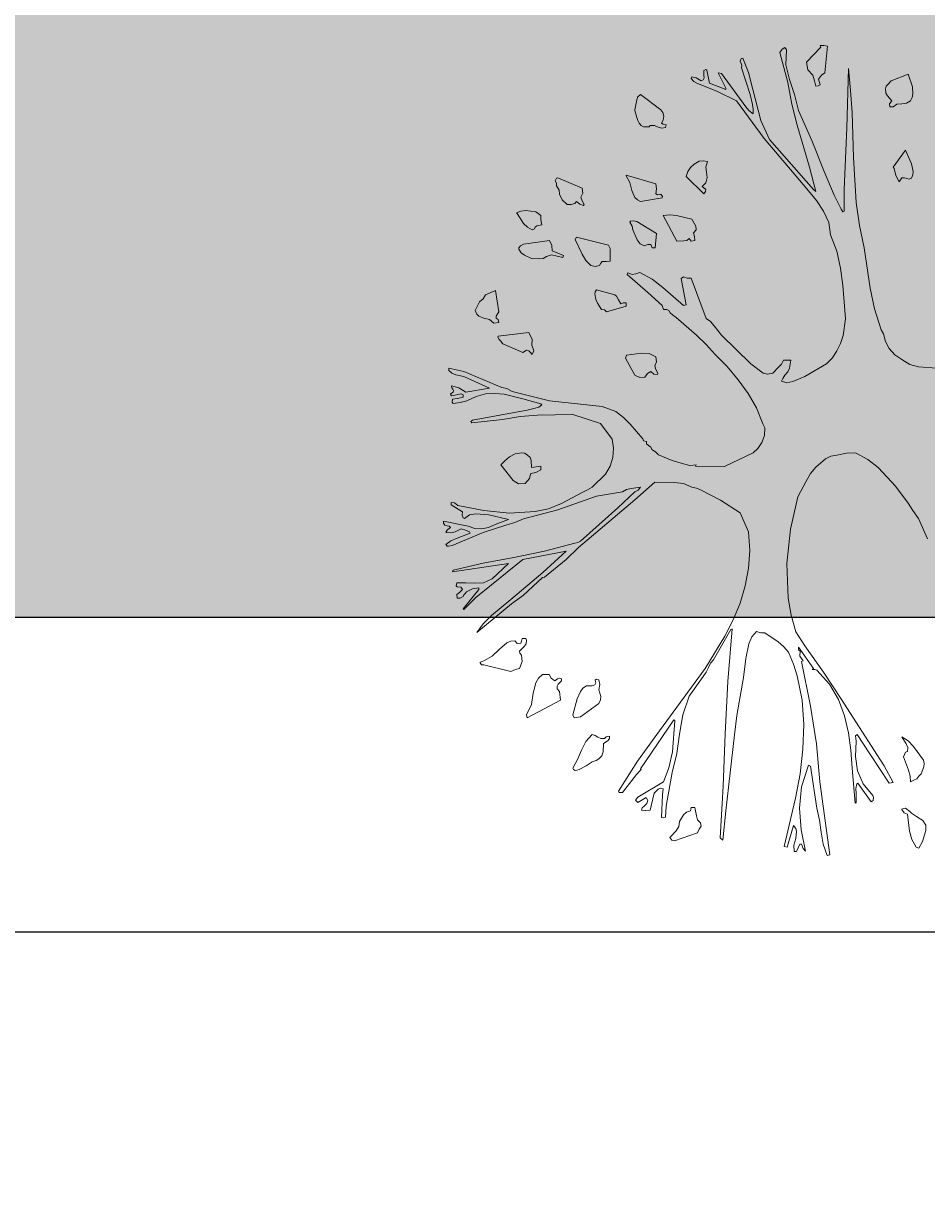
# Model space of a CAD drawing. Units: inches. Extents: x 84 to 1044, y -280 to 906.
# Tile 41 of 105: x 915 to 941, y -129 to -96. Entities that reach past the tile are written whole.
import ezdxf

# ---------------------------------------------------------------- set-up
doc = ezdxf.new("R2010")
doc.units = ezdxf.units.IN
for name, color, linetype, lineweight in [('A-ANNO-DIMS', 2, 'Continuous', 18), ('C-PROP', 7, 'Continuous', 25), ('L-PLNT', 114, 'Continuous', 15)]:
    doc.layers.add(name, color=color, linetype=linetype, lineweight=lineweight)
doc.layers.add('L-PLNT-PATT', color=9, linetype='Continuous', lineweight=9, true_color=0xafd9aa)
doc.styles.get("Standard").update_dxf_attribs({"font": 'arial.ttf'})
doc.dimstyles.get("Standard").update_dxf_attribs({"dimtxt": 0.18, "dimasz": 0.18, "dimexe": 0.18, "dimexo": 0.0625, "dimgap": 0.09, "dimtad": 0, "dimtih": 1, "dimtoh": 1, "dimdec": 4, "dimzin": 0, "dimdsep": 46, "dimtxsty": 'Standard', "dimcen": 0.09, "dimadec": 0, "dimazin": 0, "dimtfac": 1, "dimtdec": 4, "dimtofl": 0, "dimtmove": 0, "dimatfit": 3, "dimfxl": 1, "dimtolj": 1, "dimtzin": 0, "dimarcsym": 0})

# ---------------------------------------------------------------- blocks, each defined once
blk = doc.blocks.new('A$C37E508DF')
for p, q in [((0.6367, 1.5175), (0.6423, 1.5201)), ((0.6423, 1.5201), (0.6453, 1.5158)), ((0.6826, 1.493), (0.7096, 1.5209)), ((0.7083, 1.5239), (0.7152, 1.5244)), ((0.7096, 1.5209), (0.7083, 1.5239)), ((0.7152, 1.5244), (0.7225, 1.5231)), ((0.7225, 1.5231), (0.7174, 1.4729)), ((0.5583, 1.4948), (0.5596, 1.4995)), ((0.5596, 1.4995), (0.563, 1.5003)), ((0.563, 1.5003), (0.5737, 1.4733)), ((0.6329, 1.5111), (0.6367, 1.5175)), ((0.6475, 1.4545), (0.6329, 1.5111)), ((0.6453, 1.5158), (0.644, 1.4879)), ((0.4897, 1.4772), (0.4935, 1.4789)), ((0.4897, 1.4678), (0.4897, 1.4772)), ((0.4935, 1.4789), (0.4952, 1.478)), ((0.4952, 1.478), (0.5004, 1.4532)), ((0.5596, 1.4905), (0.5583, 1.4948)), ((0.5613, 1.4862), (0.5596, 1.4905)), ((0.5608, 1.4823), (0.5613, 1.4862)), ((0.5767, 1.4317), (0.5608, 1.4823)), ((0.644, 1.4879), (0.6505, 1.46)), ((0.6852, 1.4785), (0.6826, 1.493)), ((0.6946, 1.4682), (0.6852, 1.4785)), ((0.7589, 1.3691), (0.7615, 1.481)), ((0.7615, 1.481), (0.7658, 1.4395)), ((0.4657, 1.4622), (0.4669, 1.4652)), ((0.4708, 1.4566), (0.4657, 1.4622)), ((0.4669, 1.4652), (0.4755, 1.463)), ((0.4764, 1.4532), (0.4708, 1.4566)), ((0.4755, 1.463), (0.4845, 1.4575)), ((0.5154, 1.4373), (0.4764, 1.4532)), ((0.4845, 1.4575), (0.4884, 1.4596)), ((0.4884, 1.4596), (0.4905, 1.4635)), ((0.4905, 1.4635), (0.4897, 1.4678)), ((0.5004, 1.4532), (0.5308, 1.4412)), ((0.5313, 1.4437), (0.5167, 1.4729)), ((0.5167, 1.4729), (0.5231, 1.4716)), ((0.5231, 1.4716), (0.5686, 1.409)), ((0.5737, 1.4733), (0.5814, 1.4437)), ((0.6552, 1.4137), (0.6475, 1.4545)), ((0.6505, 1.46), (0.6603, 1.4317)), ((0.6976, 1.4579), (0.6946, 1.4682)), ((0.7002, 1.4476), (0.6976, 1.4579)), ((0.7109, 1.4682), (0.7053, 1.4609)), ((0.7053, 1.4609), (0.7083, 1.4502)), ((0.7174, 1.4729), (0.7109, 1.4682)), ((0.8357, 1.451), (0.8421, 1.4575)), ((0.8421, 1.4575), (0.8739, 1.4703)), ((0.8739, 1.4703), (0.882, 1.4463)), ((0.3649, 1.4266), (0.3709, 1.4317)), ((0.3709, 1.4317), (0.4086, 1.403)), ((0.551, 1.4197), (0.5154, 1.4373)), ((0.5308, 1.4412), (0.5313, 1.4437)), ((0.5814, 1.4133), (0.5767, 1.4317)), ((0.5814, 1.4437), (0.5969, 1.3833)), ((0.6603, 1.4317), (0.668, 1.4021)), ((0.7049, 1.448), (0.7002, 1.4476)), ((0.7083, 1.4502), (0.7049, 1.448)), ((0.7658, 1.4395), (0.7684, 1.3979)), ((0.831, 1.4424), (0.8323, 1.4476)), ((0.8318, 1.4343), (0.831, 1.4424)), ((0.8353, 1.4292), (0.8318, 1.4343)), ((0.8323, 1.4476), (0.8357, 1.451)), ((0.8829, 1.433), (0.8816, 1.4262)), ((0.882, 1.4463), (0.8829, 1.433)), ((0.3598, 1.403), (0.3628, 1.4189)), ((0.3628, 1.4189), (0.3649, 1.4266)), ((0.6029, 1.3494), (0.551, 1.4197)), ((0.5686, 1.409), (0.5741, 1.4021)), ((0.5827, 1.4043), (0.5814, 1.4133)), ((0.6655, 1.3743), (0.6552, 1.4137)), ((0.8434, 1.4197), (0.8353, 1.4292)), ((0.8391, 1.4141), (0.8434, 1.4197)), ((0.8395, 1.4086), (0.8391, 1.4141)), ((0.846, 1.4086), (0.8395, 1.4086)), ((0.8528, 1.4137), (0.846, 1.4086)), ((0.8619, 1.4146), (0.8528, 1.4137)), ((0.8709, 1.4154), (0.8619, 1.4146)), ((0.8781, 1.4197), (0.8709, 1.4154)), ((0.8816, 1.4262), (0.8781, 1.4197)), ((0.3602, 1.4021), (0.3598, 1.403)), ((0.364, 1.3888), (0.3602, 1.4021)), ((0.3657, 1.3828), (0.364, 1.3888)), ((0.4086, 1.403), (0.4125, 1.3979)), ((0.4125, 1.3979), (0.4142, 1.391)), ((0.4142, 1.391), (0.4134, 1.3837)), ((0.5741, 1.4021), (0.5823, 1.3953)), ((0.5823, 1.3953), (0.5827, 1.4043)), ((0.668, 1.4021), (0.6925, 1.3455)), ((0.7684, 1.3979), (0.771, 1.3134)), ((0.3683, 1.3781), (0.3657, 1.3828)), ((0.3718, 1.3738), (0.3683, 1.3781)), ((0.3765, 1.3713), (0.3718, 1.3738)), ((0.3872, 1.3708), (0.3765, 1.3713)), ((0.3885, 1.3738), (0.3872, 1.3708)), ((0.3971, 1.3734), (0.3885, 1.3738)), ((0.4039, 1.3704), (0.3971, 1.3734)), ((0.4108, 1.3683), (0.4039, 1.3704)), ((0.4134, 1.3837), (0.4099, 1.3781)), ((0.4099, 1.3781), (0.4134, 1.376)), ((0.4176, 1.37), (0.4108, 1.3683)), ((0.4134, 1.376), (0.4189, 1.3751)), ((0.4189, 1.3751), (0.4176, 1.37)), ((0.5969, 1.3833), (0.6132, 1.3472)), ((0.6882, 1.2949), (0.6655, 1.3743)), ((0.7538, 1.2529), (0.7589, 1.3691)), ((0.6595, 1.2829), (0.6029, 1.3494)), ((0.6132, 1.3472), (0.6959, 1.2529)), ((0.6925, 1.3455), (0.7161, 1.2868)), ((0.846, 1.2949), (0.8687, 1.3271)), ((0.8687, 1.3271), (0.8803, 1.3014)), ((0.4648, 1.2945), (0.4717, 1.3009)), ((0.4717, 1.3009), (0.4807, 1.3065)), ((0.4807, 1.3065), (0.4884, 1.3074)), ((0.4884, 1.3074), (0.4965, 1.3057)), ((0.4965, 1.3057), (0.4935, 1.2954)), ((0.771, 1.3134), (0.7761, 1.2285)), ((0.8803, 1.3014), (0.8833, 1.2872)), ((0.3439, 1.2804), (0.3992, 1.2636)), ((0.3439, 1.2787), (0.3439, 1.2804)), ((0.3507, 1.2662), (0.3439, 1.2787)), ((0.4562, 1.2774), (0.4597, 1.2868)), ((0.4897, 1.2452), (0.4562, 1.2774)), ((0.4597, 1.2868), (0.4648, 1.2945)), ((0.4935, 1.2954), (0.4948, 1.2855)), ((0.4948, 1.2855), (0.4961, 1.2756)), ((0.6865, 1.2508), (0.6595, 1.2829)), ((0.7002, 1.2495), (0.6882, 1.2949)), ((0.7161, 1.2868), (0.7349, 1.2422)), ((0.8473, 1.2924), (0.846, 1.2949)), ((0.8507, 1.2795), (0.8473, 1.2924)), ((0.8567, 1.2679), (0.8507, 1.2795)), ((0.8829, 1.2808), (0.8799, 1.2744)), ((0.8833, 1.2872), (0.8829, 1.2808)), ((0.2101, 1.2696), (0.2127, 1.2744)), ((0.2127, 1.2654), (0.2101, 1.2696)), ((0.2127, 1.2744), (0.2152, 1.2752)), ((0.2127, 1.2602), (0.2127, 1.2654)), ((0.2174, 1.2521), (0.2127, 1.2602)), ((0.2152, 1.2752), (0.2611, 1.2559)), ((0.2611, 1.2559), (0.262, 1.2465)), ((0.3546, 1.2516), (0.3507, 1.2662)), ((0.3992, 1.2636), (0.4005, 1.2546)), ((0.4005, 1.2546), (0.3992, 1.2452)), ((0.4935, 1.2658), (0.4867, 1.2589)), ((0.4867, 1.2589), (0.4935, 1.2529)), ((0.4961, 1.2756), (0.4935, 1.2658)), ((0.8619, 1.2752), (0.8567, 1.2679)), ((0.867, 1.2752), (0.8619, 1.2752)), ((0.8713, 1.2739), (0.867, 1.2752)), ((0.8756, 1.2726), (0.8713, 1.2739)), ((0.8799, 1.2744), (0.8756, 1.2726)), ((0.2182, 1.2443), (0.2174, 1.2521)), ((0.2234, 1.2336), (0.2182, 1.2443)), ((0.2328, 1.2251), (0.2234, 1.2336)), ((0.262, 1.2465), (0.2586, 1.2388)), ((0.2586, 1.2388), (0.2611, 1.2319)), ((0.3602, 1.2383), (0.3546, 1.2516)), ((0.3649, 1.2336), (0.3602, 1.2383)), ((0.3709, 1.2306), (0.3649, 1.2336)), ((0.4112, 1.2375), (0.3709, 1.2306)), ((0.3992, 1.2452), (0.4026, 1.2431)), ((0.4026, 1.2431), (0.4086, 1.2443)), ((0.4086, 1.2443), (0.4121, 1.2401)), ((0.4121, 1.2401), (0.4112, 1.2375)), ((0.4931, 1.2491), (0.4897, 1.2452)), ((0.4935, 1.2529), (0.4931, 1.2491)), ((0.7015, 1.2323), (0.6865, 1.2508)), ((0.6959, 1.2529), (0.7002, 1.2495)), ((0.7148, 1.2126), (0.7015, 1.2323)), ((0.7349, 1.2422), (0.7482, 1.216)), ((0.7538, 1.2122), (0.7538, 1.2529)), ((0.1376, 1.2092), (0.1458, 1.2126)), ((0.1458, 1.2126), (0.1548, 1.2135)), ((0.1548, 1.2135), (0.1741, 1.2109)), ((0.1741, 1.2109), (0.1784, 1.2083)), ((0.2401, 1.2251), (0.2328, 1.2251)), ((0.2474, 1.2268), (0.2401, 1.2251)), ((0.2504, 1.2306), (0.2474, 1.2268)), ((0.2568, 1.2255), (0.2504, 1.2306)), ((0.2633, 1.2229), (0.2568, 1.2255)), ((0.2611, 1.2319), (0.265, 1.2251)), ((0.265, 1.2251), (0.2633, 1.2229)), ((0.7246, 1.1908), (0.7148, 1.2126)), ((0.7482, 1.216), (0.7508, 1.2109)), ((0.7508, 1.2109), (0.7538, 1.2122)), ((0.7761, 1.2285), (0.7821, 1.1856)), ((0.1389, 1.2079), (0.1376, 1.2092)), ((0.1505, 1.189), (0.1389, 1.2079)), ((0.1582, 1.1822), (0.1505, 1.189)), ((0.1784, 1.2083), (0.1831, 1.204)), ((0.1831, 1.204), (0.1831, 1.1959)), ((0.1831, 1.1959), (0.1848, 1.1865)), ((0.3507, 1.1916), (0.352, 1.1933)), ((0.355, 1.1839), (0.3507, 1.1916)), ((0.352, 1.1933), (0.3576, 1.1942)), ((0.3576, 1.1942), (0.364, 1.1929)), ((0.364, 1.1929), (0.4005, 1.1702)), ((0.4134, 1.204), (0.4258, 1.2058)), ((0.4391, 1.156), (0.4134, 1.204)), ((0.4258, 1.2058), (0.4382, 1.2045)), ((0.4382, 1.2045), (0.4669, 1.1972)), ((0.4669, 1.1972), (0.4747, 1.1843)), ((0.7281, 1.168), (0.7246, 1.1908)), ((0.1668, 1.1775), (0.1582, 1.1822)), ((0.1711, 1.1792), (0.1668, 1.1775)), ((0.1728, 1.1826), (0.1711, 1.1792)), ((0.1758, 1.1847), (0.1728, 1.1826)), ((0.1788, 1.1852), (0.1758, 1.1847)), ((0.1848, 1.1865), (0.1788, 1.1852)), ((0.3563, 1.177), (0.355, 1.1839)), ((0.3645, 1.1586), (0.3563, 1.177)), ((0.4005, 1.1702), (0.3979, 1.1436)), ((0.4751, 1.177), (0.47, 1.1714)), ((0.47, 1.1714), (0.4721, 1.1646)), ((0.4747, 1.1843), (0.4751, 1.177)), ((0.7396, 1.1371), (0.7281, 1.168)), ((0.7821, 1.1856), (0.7911, 1.1436)), ((0.1419, 1.1436), (0.1449, 1.1474)), ((0.1449, 1.1474), (0.1509, 1.1504)), ((0.1509, 1.1504), (0.1994, 1.1573)), ((0.1994, 1.1573), (0.2041, 1.1479)), ((0.2041, 1.1479), (0.2045, 1.138)), ((0.2478, 1.1594), (0.2504, 1.1637)), ((0.2607, 1.1316), (0.2478, 1.1594)), ((0.2504, 1.1637), (0.3104, 1.1487)), ((0.3104, 1.1487), (0.3134, 1.1423)), ((0.37, 1.1509), (0.3645, 1.1586)), ((0.3778, 1.1474), (0.37, 1.1509)), ((0.3842, 1.15), (0.3778, 1.1474)), ((0.3898, 1.15), (0.3842, 1.15)), ((0.3923, 1.1436), (0.3898, 1.15)), ((0.4519, 1.1564), (0.4391, 1.156)), ((0.458, 1.1573), (0.4519, 1.1564)), ((0.4622, 1.1607), (0.458, 1.1573)), ((0.4657, 1.156), (0.4622, 1.1607)), ((0.473, 1.1573), (0.4657, 1.156)), ((0.4721, 1.1646), (0.473, 1.1573)), ((0.1419, 1.141), (0.1419, 1.1436)), ((0.1462, 1.1342), (0.1419, 1.141)), ((0.1522, 1.1294), (0.1462, 1.1342)), ((0.1655, 1.1234), (0.1522, 1.1294)), ((0.181, 1.1226), (0.1655, 1.1234)), ((0.1878, 1.1234), (0.181, 1.1226)), ((0.1938, 1.1273), (0.1878, 1.1234)), ((0.2032, 1.1303), (0.1938, 1.1273)), ((0.2247, 1.1251), (0.2032, 1.1303)), ((0.2045, 1.138), (0.226, 1.129)), ((0.226, 1.129), (0.2247, 1.1251)), ((0.268, 1.1196), (0.2607, 1.1316)), ((0.3134, 1.1423), (0.3139, 1.1346)), ((0.3139, 1.1346), (0.3134, 1.1183)), ((0.3979, 1.1436), (0.3923, 1.1436)), ((0.7469, 1.1054), (0.7396, 1.1371)), ((0.7911, 1.1436), (0.8027, 1.0677)), ((0.277, 1.1101), (0.268, 1.1196)), ((0.2856, 1.108), (0.277, 1.1101)), ((0.2933, 1.1101), (0.2856, 1.108)), ((0.2959, 1.1144), (0.2933, 1.1101)), ((0.2984, 1.1179), (0.2959, 1.1144)), ((0.3066, 1.1179), (0.2984, 1.1179)), ((0.3134, 1.1183), (0.3066, 1.1179)), ((0.7512, 1.0728), (0.7469, 1.1054)), ((0.3456, 1.093), (0.3469, 1.0964)), ((0.3842, 1.0591), (0.3456, 1.093)), ((0.3469, 1.0964), (0.355, 1.093)), ((0.355, 1.093), (0.3619, 1.0943)), ((0.3619, 1.0943), (0.3692, 1.0968)), ((0.3692, 1.0968), (0.3923, 1.0844)), ((0.3923, 1.0844), (0.4129, 1.069)), ((0.4472, 1.0857), (0.4515, 1.0887)), ((0.4562, 1.0364), (0.4472, 1.0857)), ((0.4515, 1.0887), (0.4584, 1.0865)), ((0.4584, 1.0865), (0.4657, 1.0861)), ((0.4657, 1.0861), (0.4939, 1.0107)), ((0.0789, 1.0552), (0.0978, 1.063)), ((0.0978, 1.063), (0.1042, 1.0231)), ((0.2847, 1.0565), (0.2856, 1.0604)), ((0.2851, 1.054), (0.2847, 1.0565)), ((0.2856, 1.0604), (0.2877, 1.0647)), ((0.2877, 1.0647), (0.3224, 1.0552)), ((0.4112, 1.0351), (0.3842, 1.0591)), ((0.4129, 1.069), (0.4515, 1.0351)), ((0.7538, 1.0415), (0.7512, 1.0728)), ((0.8027, 1.0677), (0.8108, 1.0287)), ((0.0596, 1.0257), (0.0682, 1.0415)), ((0.0682, 1.0415), (0.0746, 1.0475)), ((0.0746, 1.0475), (0.0789, 1.0552)), ((0.2864, 1.0463), (0.2851, 1.054)), ((0.2899, 1.039), (0.2864, 1.0463)), ((0.2972, 1.0274), (0.2899, 1.039)), ((0.3224, 1.0552), (0.3255, 1.0522)), ((0.3255, 1.0522), (0.3293, 1.0458)), ((0.3293, 1.0458), (0.3336, 1.0381)), ((0.3336, 1.0381), (0.3383, 1.0398)), ((0.3383, 1.0398), (0.3439, 1.0402)), ((0.3439, 1.0402), (0.3439, 1.0338)), ((0.4138, 1.0274), (0.4112, 1.0351)), ((0.4515, 1.0351), (0.4562, 1.0364)), ((0.7559, 1.0098), (0.7538, 1.0415)), ((0.0626, 1.0188), (0.0596, 1.0257)), ((0.0665, 1.0149), (0.0626, 1.0188)), ((0.0763, 1.0111), (0.0665, 1.0149)), ((0.1012, 1.018), (0.099, 1.0149)), ((0.099, 1.0149), (0.099, 1.0111)), ((0.1042, 1.0231), (0.1012, 1.018)), ((0.3032, 1.0265), (0.2972, 1.0274)), ((0.3066, 1.0231), (0.3032, 1.0265)), ((0.3439, 1.0338), (0.3066, 1.0231)), ((0.4202, 1.0274), (0.4138, 1.0274)), ((0.4241, 1.0257), (0.4202, 1.0274)), ((0.4267, 1.0209), (0.4241, 1.0257)), ((0.4305, 1.0175), (0.4267, 1.0209)), ((0.4378, 1.0124), (0.4305, 1.0175)), ((0.476, 0.9789), (0.4378, 1.0124)), ((0.8108, 1.0287), (0.8233, 0.9892)), ((0.087, 1.0085), (0.0763, 1.0111)), ((0.0948, 1.0016), (0.087, 1.0085)), ((0.1042, 1.0029), (0.0948, 1.0016)), ((0.099, 1.0111), (0.1033, 1.0085)), ((0.1033, 1.0085), (0.1042, 1.0029)), ((0.4939, 1.0107), (0.5021, 1.0051)), ((0.5021, 1.0051), (0.5094, 0.9969)), ((0.5094, 0.9969), (0.5231, 0.9789)), ((0.7516, 0.9785), (0.7559, 1.0098)), ((0.1025, 0.9751), (0.1029, 0.9772)), ((0.1046, 0.9708), (0.1025, 0.9751)), ((0.1029, 0.9772), (0.1604, 0.9841)), ((0.1076, 0.9682), (0.1046, 0.9708)), ((0.1119, 0.9626), (0.1076, 0.9682)), ((0.1604, 0.9841), (0.1672, 0.9708)), ((0.1672, 0.9708), (0.1664, 0.9601)), ((0.4939, 0.9618), (0.476, 0.9789)), ((0.5231, 0.9789), (0.578, 0.9253)), ((0.7469, 0.9635), (0.7516, 0.9785)), ((0.8233, 0.9892), (0.8275, 0.9815)), ((0.8275, 0.9815), (0.8314, 0.9673)), ((0.1496, 0.9463), (0.1119, 0.9626)), ((0.1565, 0.9506), (0.1496, 0.9463)), ((0.1604, 0.9493), (0.1565, 0.9506)), ((0.1629, 0.9468), (0.1604, 0.9493)), ((0.1672, 0.9429), (0.1629, 0.9468)), ((0.1664, 0.9601), (0.1698, 0.9493)), ((0.1698, 0.9493), (0.1672, 0.9429)), ((0.5111, 0.9429), (0.4939, 0.9618)), ((0.7315, 0.9365), (0.7401, 0.9493)), ((0.7401, 0.9493), (0.7469, 0.9635)), ((0.8314, 0.9673), (0.8383, 0.954)), ((0.8383, 0.954), (0.8486, 0.942)), ((0.3426, 0.936), (0.3443, 0.9412)), ((0.3602, 0.9039), (0.3426, 0.936)), ((0.3443, 0.9412), (0.3722, 0.9451)), ((0.3722, 0.9451), (0.3868, 0.9446)), ((0.3868, 0.9446), (0.3992, 0.9386)), ((0.4009, 0.9292), (0.3975, 0.9215)), ((0.3992, 0.9386), (0.4009, 0.9292)), ((0.5334, 0.9202), (0.5111, 0.9429)), ((0.578, 0.9253), (0.6011, 0.9077)), ((0.6303, 0.9189), (0.6359, 0.9245)), ((0.6359, 0.9245), (0.6397, 0.9322)), ((0.6397, 0.9322), (0.653, 0.9322)), ((0.653, 0.9322), (0.6505, 0.9172)), ((0.6796, 0.9013), (0.7203, 0.9253)), ((0.7203, 0.9253), (0.7315, 0.9365)), ((0.8486, 0.942), (0.8619, 0.933)), ((0.8619, 0.933), (0.8769, 0.9236)), ((0.0103, 0.9129), (0.0103, 0.9172)), ((0.0103, 0.9172), (0.0382, 0.9107)), ((0.0159, 0.9073), (0.0103, 0.9129)), ((0.0232, 0.9043), (0.0159, 0.9073)), ((0.0386, 0.9013), (0.0232, 0.9043)), ((0.0382, 0.9107), (0.1098, 0.8807)), ((0.3692, 0.8992), (0.3602, 0.9039)), ((0.3838, 0.9069), (0.379, 0.9)), ((0.3898, 0.9107), (0.3838, 0.9069)), ((0.3958, 0.906), (0.3898, 0.9107)), ((0.4026, 0.9052), (0.3958, 0.906)), ((0.3975, 0.9215), (0.3996, 0.9142)), ((0.3996, 0.9142), (0.4031, 0.9077)), ((0.4031, 0.9077), (0.4026, 0.9052)), ((0.554, 0.8953), (0.5334, 0.9202)), ((0.6011, 0.9077), (0.6097, 0.9056)), ((0.6097, 0.9056), (0.6196, 0.9077)), ((0.6196, 0.9077), (0.6303, 0.9189)), ((0.6423, 0.9039), (0.6384, 0.8974)), ((0.6479, 0.9103), (0.6423, 0.9039)), ((0.6505, 0.9172), (0.6479, 0.9103)), ((0.8769, 0.9236), (0.8936, 0.9193)), ((0.8936, 0.9193), (0.9279, 0.9172)), ((0.0159, 0.8803), (0.0154, 0.8837)), ((0.0154, 0.8837), (0.0292, 0.8803)), ((0.0176, 0.8777), (0.0159, 0.8803)), ((0.0292, 0.8803), (0.0424, 0.8717)), ((0.0866, 0.8794), (0.0386, 0.9013)), ((0.1098, 0.8807), (0.1196, 0.8786)), ((0.379, 0.9), (0.3692, 0.8992)), ((0.5728, 0.8691), (0.554, 0.8953)), ((0.6384, 0.8974), (0.6359, 0.8927)), ((0.6359, 0.8927), (0.6457, 0.8897)), ((0.6457, 0.8897), (0.6569, 0.8919)), ((0.6569, 0.8919), (0.6796, 0.9013)), ((0.0133, 0.8679), (0.015, 0.87)), ((0.0154, 0.8649), (0.0133, 0.8679)), ((0.015, 0.87), (0.0184, 0.8717)), ((0.0334, 0.8687), (0.0154, 0.8649)), ((0.0163, 0.8529), (0.0171, 0.8584)), ((0.0171, 0.8584), (0.0266, 0.8602)), ((0.0193, 0.8752), (0.0176, 0.8777)), ((0.0184, 0.8717), (0.0193, 0.8752)), ((0.0266, 0.8602), (0.0369, 0.8623)), ((0.0369, 0.8666), (0.0334, 0.8687)), ((0.0369, 0.8623), (0.0369, 0.8666)), ((0.0424, 0.8717), (0.0866, 0.8794)), ((0.0617, 0.864), (0.0442, 0.8554)), ((0.0789, 0.8687), (0.0617, 0.864)), ((0.0965, 0.8696), (0.0789, 0.8687)), ((0.1141, 0.8679), (0.0965, 0.8696)), ((0.1492, 0.8593), (0.1141, 0.8679)), ((0.1196, 0.8786), (0.1295, 0.873)), ((0.1295, 0.873), (0.1994, 0.8554)), ((0.1835, 0.8499), (0.1492, 0.8593)), ((0.5887, 0.8421), (0.5728, 0.8691)), ((0.0184, 0.8503), (0.0163, 0.8529)), ((0.0317, 0.8524), (0.0184, 0.8503)), ((0.0442, 0.8554), (0.0317, 0.8524)), ((0.0545, 0.8194), (0.1578, 0.8378)), ((0.1578, 0.8378), (0.1698, 0.8413)), ((0.1698, 0.8413), (0.1792, 0.8434)), ((0.1792, 0.8434), (0.1848, 0.8477)), ((0.1848, 0.8477), (0.1835, 0.8499)), ((0.1994, 0.8554), (0.2984, 0.8447)), ((0.2984, 0.8447), (0.3242, 0.8357)), ((0.6007, 0.8125), (0.5887, 0.8421)), ((0.0519, 0.8164), (0.0545, 0.8194)), ((0.0532, 0.8143), (0.0519, 0.8164)), ((0.1111, 0.8207), (0.0532, 0.8143)), ((0.1441, 0.8258), (0.1111, 0.8207)), ((0.1771, 0.8288), (0.1441, 0.8258)), ((0.2436, 0.8301), (0.1771, 0.8288)), ((0.2954, 0.813), (0.2436, 0.8301)), ((0.3242, 0.8357), (0.3387, 0.8241)), ((0.3387, 0.8241), (0.3512, 0.8117)), ((0.3173, 0.7834), (0.2954, 0.813)), ((0.3512, 0.8117), (0.3748, 0.7842)), ((0.6046, 0.8048), (0.6007, 0.8125)), ((0.6037, 0.7903), (0.6046, 0.8048)), ((0.3199, 0.7662), (0.3173, 0.7834)), ((0.3748, 0.7842), (0.3765, 0.7804)), ((0.3765, 0.7804), (0.3816, 0.7791)), ((0.3816, 0.7791), (0.382, 0.7744)), ((0.382, 0.7744), (0.3859, 0.7714)), ((0.3859, 0.7714), (0.3902, 0.7684)), ((0.5913, 0.7658), (0.599, 0.777)), ((0.599, 0.777), (0.6037, 0.7903)), ((0.1153, 0.7427), (0.1244, 0.7504)), ((0.1244, 0.7504), (0.1351, 0.7559)), ((0.1351, 0.7559), (0.1471, 0.7577)), ((0.1471, 0.7577), (0.1527, 0.7568)), ((0.1527, 0.7568), (0.1578, 0.7538)), ((0.1578, 0.7538), (0.1629, 0.7491)), ((0.1629, 0.7491), (0.1651, 0.7431)), ((0.3139, 0.7324), (0.3186, 0.7491)), ((0.3186, 0.7491), (0.3199, 0.7662)), ((0.3902, 0.7684), (0.3919, 0.7641)), ((0.3919, 0.7641), (0.3988, 0.7598)), ((0.3988, 0.7598), (0.4043, 0.7538)), ((0.4043, 0.7538), (0.4301, 0.7431)), ((0.5287, 0.7319), (0.5823, 0.7577)), ((0.5823, 0.7577), (0.5913, 0.7658)), ((0.7285, 0.7512), (0.7182, 0.7461)), ((0.7401, 0.7534), (0.7285, 0.7512)), ((0.7577, 0.7568), (0.7401, 0.7534)), ((0.7752, 0.7577), (0.7577, 0.7568)), ((0.798, 0.7452), (0.7752, 0.7577)), ((0.1081, 0.7349), (0.1153, 0.7427)), ((0.1312, 0.7058), (0.1081, 0.7349)), ((0.1651, 0.7431), (0.1655, 0.7298)), ((0.1655, 0.7298), (0.1831, 0.7324)), ((0.1831, 0.7324), (0.1831, 0.7255)), ((0.3049, 0.7178), (0.3139, 0.7324)), ((0.4301, 0.7431), (0.4515, 0.7371)), ((0.4515, 0.7371), (0.4635, 0.7341)), ((0.4635, 0.7341), (0.4755, 0.7349)), ((0.4755, 0.7349), (0.4742, 0.7324)), ((0.4742, 0.7324), (0.5287, 0.7319)), ((0.7002, 0.7307), (0.6903, 0.7186)), ((0.7182, 0.7461), (0.7002, 0.7307)), ((0.8173, 0.7298), (0.798, 0.7452)), ((0.8344, 0.7122), (0.8173, 0.7298)), ((0.1415, 0.6994), (0.1312, 0.7058)), ((0.1621, 0.7092), (0.1539, 0.7002)), ((0.1629, 0.7152), (0.1621, 0.7092)), ((0.1646, 0.7186), (0.1629, 0.7152)), ((0.1741, 0.7208), (0.1646, 0.7186)), ((0.1831, 0.7255), (0.1741, 0.7208)), ((0.28, 0.6933), (0.3049, 0.7178)), ((0.6903, 0.7186), (0.6818, 0.7032)), ((0.8503, 0.6951), (0.8344, 0.7122)), ((0.1539, 0.7002), (0.1415, 0.6994)), ((0.2221, 0.6625), (0.262, 0.6839)), ((0.262, 0.6839), (0.271, 0.6882)), ((0.271, 0.6882), (0.28, 0.6933)), ((0.337, 0.6843), (0.2877, 0.6762)), ((0.328, 0.6543), (0.3598, 0.6843)), ((0.3443, 0.6886), (0.337, 0.6843)), ((0.3533, 0.6903), (0.3443, 0.6886)), ((0.3709, 0.6933), (0.3533, 0.6903)), ((0.3975, 0.7028), (0.3598, 0.6693)), ((0.3598, 0.6843), (0.3662, 0.6873)), ((0.3662, 0.6873), (0.3709, 0.6933)), ((0.4339, 0.7019), (0.3975, 0.7028)), ((0.4515, 0.7002), (0.4339, 0.7019)), ((0.4674, 0.6933), (0.4515, 0.7002)), ((0.476, 0.6912), (0.4674, 0.6933)), ((0.4832, 0.6878), (0.476, 0.6912)), ((0.521, 0.6685), (0.4832, 0.6878)), ((0.6818, 0.7032), (0.6667, 0.6749)), ((0.8739, 0.6629), (0.8503, 0.6951)), ((0.0146, 0.6599), (0.0146, 0.6642)), ((0.0146, 0.6642), (0.0206, 0.6633)), ((0.0206, 0.6633), (0.0274, 0.6586)), ((0.1977, 0.6526), (0.2221, 0.6625)), ((0.2877, 0.6762), (0.2152, 0.6505)), ((0.3598, 0.6693), (0.2543, 0.5797)), ((0.5578, 0.6449), (0.521, 0.6685)), ((0.6667, 0.6749), (0.6526, 0.614)), ((0.8824, 0.6492), (0.8739, 0.6629)), ((0.036, 0.6466), (0.0146, 0.6599)), ((0.0274, 0.6586), (0.0759, 0.6492)), ((0.0356, 0.6406), (0.036, 0.6466)), ((0.0369, 0.6355), (0.0356, 0.6406)), ((0.0489, 0.641), (0.0399, 0.6342)), ((0.0609, 0.6428), (0.0489, 0.641)), ((0.0853, 0.641), (0.0609, 0.6428)), ((0.0759, 0.6492), (0.1244, 0.644)), ((0.1226, 0.632), (0.0853, 0.641)), ((0.1244, 0.644), (0.1728, 0.647)), ((0.2152, 0.6505), (0.1509, 0.6333)), ((0.1728, 0.647), (0.1977, 0.6526)), ((0.2581, 0.5913), (0.328, 0.6543)), ((0.5737, 0.6089), (0.5578, 0.6449)), ((0.8932, 0.6342), (0.8824, 0.6492)), ((0, 0.629), (0.0467, 0.62)), ((0, 0.6252), (0, 0.629)), ((0.003, 0.6213), (0, 0.6252)), ((0.0069, 0.6204), (0.003, 0.6213)), ((0.0107, 0.6196), (0.0069, 0.6204)), ((0.0086, 0.6132), (0.0133, 0.617)), ((0.0133, 0.617), (0.0107, 0.6196)), ((0.0399, 0.6342), (0.0369, 0.6355)), ((0.0467, 0.62), (0.0592, 0.6153)), ((0.072, 0.6149), (0.0849, 0.6175)), ((0.1175, 0.6213), (0.0746, 0.6076)), ((0.0849, 0.6175), (0.0973, 0.6226)), ((0.0973, 0.6226), (0.1226, 0.632)), ((0.1342, 0.6265), (0.1175, 0.6213)), ((0.1509, 0.6333), (0.1342, 0.6265)), ((0.9103, 0.5956), (0.8932, 0.6342)), ((0.0047, 0.6093), (0.0086, 0.6132)), ((0.0056, 0.6076), (0.0047, 0.6093)), ((0.0141, 0.6072), (0.0056, 0.6076)), ((0.0223, 0.6089), (0.0141, 0.6072)), ((0.0141, 0.5921), (0.0257, 0.5969)), ((0.0746, 0.6076), (0.0163, 0.5836)), ((0.0334, 0.6145), (0.0223, 0.6089)), ((0.0257, 0.5969), (0.0506, 0.6063)), ((0.0416, 0.6119), (0.0334, 0.6145)), ((0.0493, 0.6093), (0.0416, 0.6119)), ((0.0506, 0.6063), (0.0493, 0.6093)), ((0.0592, 0.6153), (0.072, 0.6149)), ((0.5763, 0.5741), (0.5737, 0.6089)), ((0.6526, 0.614), (0.6457, 0.5497)), ((0.0047, 0.5849), (0.0141, 0.5921)), ((0.0069, 0.5823), (0.0047, 0.5849)), ((0.0099, 0.5823), (0.0069, 0.5823)), ((0.0163, 0.5836), (0.0099, 0.5823)), ((0.1325, 0.5608), (0.1904, 0.5724)), ((0.2311, 0.5729), (0.1496, 0.557)), ((0.1869, 0.5325), (0.2311, 0.5729)), ((0.1904, 0.5724), (0.2474, 0.5879)), ((0.2543, 0.5797), (0.2311, 0.557)), ((0.2474, 0.5879), (0.253, 0.5892)), ((0.253, 0.5892), (0.2581, 0.5913)), ((0.5737, 0.5407), (0.5763, 0.5741)), ((0.0184, 0.5368), (0.0746, 0.5501)), ((0.1496, 0.557), (0.0613, 0.4858)), ((0.0746, 0.5501), (0.1325, 0.5608)), ((0.2311, 0.557), (0.1899, 0.5235)), ((0.1226, 0.5497), (0.0171, 0.5338)), ((0.0171, 0.5338), (0.0184, 0.5368)), ((0.0917, 0.5205), (0.1226, 0.5497)), ((0.1269, 0.482), (0.1869, 0.5325)), ((0.5677, 0.5077), (0.5737, 0.5407)), ((0.6457, 0.5497), (0.6483, 0.4845)), ((0.024, 0.5072), (0.0253, 0.5128)), ((0.0262, 0.5055), (0.024, 0.5072)), ((0.0253, 0.5128), (0.042, 0.5133)), ((0.042, 0.5133), (0.0587, 0.5124)), ((0.0587, 0.5124), (0.0755, 0.5133)), ((0.0755, 0.5133), (0.0917, 0.5205)), ((0.1861, 0.5231), (0.1509, 0.4897)), ((0.1899, 0.5235), (0.1861, 0.5231)), ((0.5578, 0.4751), (0.5677, 0.5077)), ((0.0253, 0.491), (0.03, 0.4948)), ((0.0262, 0.4841), (0.0253, 0.491)), ((0.0326, 0.5047), (0.0262, 0.5055)), ((0.0317, 0.4841), (0.0262, 0.4841)), ((0.03, 0.4948), (0.036, 0.5004)), ((0.0369, 0.4871), (0.0317, 0.4841)), ((0.036, 0.5004), (0.0326, 0.5047)), ((0.0369, 0.4639), (0.0669, 0.5004)), ((0.0382, 0.4905), (0.0369, 0.4871)), ((0.0403, 0.4922), (0.0382, 0.4905)), ((0.0613, 0.4858), (0.0386, 0.4627)), ((0.0437, 0.4961), (0.0403, 0.4922)), ((0.0549, 0.5021), (0.0437, 0.4961)), ((0.0669, 0.5034), (0.0549, 0.5021)), ((0.0669, 0.5004), (0.0669, 0.5034)), ((0.1509, 0.4897), (0.1282, 0.4734)), ((0.6483, 0.4845), (0.6539, 0.4524)), ((0.0386, 0.4627), (0.0369, 0.4639)), ((0.1282, 0.4734), (0.0626, 0.4198)), ((0.0905, 0.4515), (0.1269, 0.482)), ((0.545, 0.4434), (0.5578, 0.4751)), ((0.0746, 0.4361), (0.0905, 0.4515)), ((0.5295, 0.4125), (0.545, 0.4434)), ((0.6539, 0.4524), (0.6625, 0.4211)), ((0.0626, 0.4198), (0.0746, 0.4361)), ((0.5403, 0.4254), (0.5081, 0.3679)), ((0.5347, 0.3276), (0.5433, 0.4266)), ((0.5433, 0.4266), (0.5403, 0.4254)), ((0.5887, 0.4215), (0.5797, 0.4112)), ((0.5969, 0.4189), (0.5887, 0.4215)), ((0.6046, 0.4189), (0.5969, 0.4189)), ((0.6295, 0.4022), (0.6046, 0.4189)), ((0.6625, 0.4211), (0.6796, 0.3945)), ((0.1055, 0.388), (0.1192, 0.4001)), ((0.1192, 0.4001), (0.1265, 0.4031)), ((0.1265, 0.4031), (0.1346, 0.4039)), ((0.1346, 0.4039), (0.1389, 0.3992)), ((0.1389, 0.3992), (0.1458, 0.3996)), ((0.1458, 0.3996), (0.1471, 0.4035)), ((0.1471, 0.4035), (0.1484, 0.4082)), ((0.1484, 0.4082), (0.1548, 0.4082)), ((0.1556, 0.3983), (0.1518, 0.3932)), ((0.1548, 0.4082), (0.1565, 0.4052)), ((0.1565, 0.4052), (0.1556, 0.3983)), ((0.4922, 0.3516), (0.5295, 0.4125)), ((0.5741, 0.3983), (0.5686, 0.3705)), ((0.5797, 0.4112), (0.5741, 0.3983)), ((0.6397, 0.3936), (0.6295, 0.4022)), ((0.0763, 0.3662), (0.0917, 0.3748)), ((0.0917, 0.3748), (0.1055, 0.388)), ((0.1518, 0.3932), (0.1432, 0.3842)), ((0.1432, 0.3842), (0.1436, 0.3808)), ((0.1436, 0.3808), (0.1471, 0.3769)), ((0.1471, 0.3769), (0.1484, 0.3649)), ((0.6487, 0.3825), (0.6397, 0.3936)), ((0.6582, 0.3602), (0.6487, 0.3825)), ((0.6959, 0.352), (0.668, 0.3919)), ((0.668, 0.3919), (0.668, 0.3872)), ((0.668, 0.3872), (0.6706, 0.3842)), ((0.6706, 0.3842), (0.6702, 0.3748)), ((0.6702, 0.3748), (0.6762, 0.3662)), ((0.6796, 0.3945), (0.7148, 0.3447)), ((0.069, 0.364), (0.0763, 0.3662)), ((0.069, 0.3627), (0.069, 0.364)), ((0.0716, 0.3585), (0.069, 0.3627)), ((0.0763, 0.3585), (0.0716, 0.3585)), ((0.1269, 0.3464), (0.0763, 0.3585)), ((0.1432, 0.352), (0.1355, 0.3499)), ((0.1484, 0.3649), (0.1432, 0.352)), ((0.4982, 0.3537), (0.4939, 0.3447)), ((0.5025, 0.3619), (0.4982, 0.3537)), ((0.5081, 0.3679), (0.5025, 0.3619)), ((0.5686, 0.3705), (0.5643, 0.3349)), ((0.665, 0.3379), (0.6582, 0.3602)), ((0.6762, 0.3662), (0.6732, 0.3653)), ((0.6732, 0.3653), (0.6903, 0.2813)), ((0.6933, 0.3503), (0.6959, 0.352)), ((0.1355, 0.3499), (0.1269, 0.3464)), ((0.1737, 0.325), (0.1788, 0.3336)), ((0.1788, 0.3336), (0.1861, 0.3409)), ((0.1861, 0.3409), (0.199, 0.3409)), ((0.199, 0.3409), (0.2024, 0.3336)), ((0.2024, 0.3336), (0.2097, 0.3289)), ((0.2097, 0.3289), (0.2148, 0.3323)), ((0.2148, 0.3323), (0.2182, 0.3336)), ((0.2182, 0.3336), (0.2221, 0.3327)), ((0.2221, 0.3327), (0.2221, 0.3289)), ((0.2851, 0.3302), (0.2877, 0.3319)), ((0.2864, 0.325), (0.2851, 0.3302)), ((0.2877, 0.3319), (0.292, 0.3306)), ((0.292, 0.3306), (0.2941, 0.322)), ((0.4065, 0.2345), (0.4922, 0.3516)), ((0.4884, 0.337), (0.4622, 0.2997)), ((0.4939, 0.3447), (0.4884, 0.337)), ((0.5643, 0.3349), (0.5578, 0.2993)), ((0.6745, 0.2924), (0.665, 0.3379)), ((0.6985, 0.3503), (0.6933, 0.3503)), ((0.7023, 0.349), (0.6985, 0.3503)), ((0.7259, 0.3224), (0.7023, 0.349)), ((0.7148, 0.3447), (0.7487, 0.2937)), ((0.1689, 0.3053), (0.1737, 0.325)), ((0.2161, 0.3224), (0.214, 0.3186)), ((0.214, 0.3186), (0.214, 0.3139)), ((0.214, 0.3139), (0.2182, 0.3087)), ((0.2221, 0.3289), (0.2161, 0.3224)), ((0.2182, 0.3087), (0.2204, 0.292)), ((0.2517, 0.2946), (0.2577, 0.3087)), ((0.2577, 0.3087), (0.2624, 0.3147)), ((0.2624, 0.3147), (0.2689, 0.3194)), ((0.2689, 0.3194), (0.2796, 0.3194)), ((0.2796, 0.3194), (0.2847, 0.3211)), ((0.2847, 0.3211), (0.2864, 0.325)), ((0.2941, 0.322), (0.292, 0.3117)), ((0.292, 0.3117), (0.2959, 0.2993)), ((0.53, 0.229), (0.5347, 0.3276)), ((0.7427, 0.2937), (0.7259, 0.3224)), ((0.2204, 0.292), (0.1578, 0.259)), ((0.1655, 0.2843), (0.1689, 0.3053)), ((0.2436, 0.265), (0.2517, 0.2946)), ((0.2954, 0.2928), (0.292, 0.286)), ((0.2959, 0.2993), (0.2954, 0.2928)), ((0.4622, 0.2997), (0.4502, 0.2645)), ((0.5578, 0.2993), (0.5518, 0.2633)), ((0.6775, 0.2465), (0.6745, 0.2924)), ((0.7542, 0.2628), (0.7427, 0.2937)), ((0.7487, 0.2937), (0.8151, 0.1899)), ((0.1565, 0.265), (0.1655, 0.2843)), ((0.1578, 0.259), (0.1565, 0.265)), ((0.2461, 0.259), (0.2436, 0.265)), ((0.292, 0.286), (0.2581, 0.2607)), ((0.4502, 0.2645), (0.4438, 0.2285)), ((0.6903, 0.2813), (0.7015, 0.2101)), ((0.2581, 0.2607), (0.2461, 0.259)), ((0.4335, 0.2556), (0.3709, 0.1634)), ((0.4305, 0.1951), (0.4352, 0.2543)), ((0.4352, 0.2543), (0.4335, 0.2556)), ((0.5518, 0.2633), (0.5475, 0.2268)), ((0.6758, 0.2002), (0.6775, 0.2465)), ((0.7615, 0.2311), (0.7542, 0.2628)), ((0.268, 0.2148), (0.28, 0.2277)), ((0.28, 0.2277), (0.2851, 0.226)), ((0.2851, 0.226), (0.2903, 0.2225)), ((0.2903, 0.2225), (0.2963, 0.22)), ((0.2963, 0.22), (0.3027, 0.2204)), ((0.3027, 0.2204), (0.3061, 0.2234)), ((0.3061, 0.2234), (0.3122, 0.2247)), ((0.3122, 0.2247), (0.3122, 0.22)), ((0.3649, 0.1775), (0.4065, 0.2345)), ((0.4438, 0.2285), (0.4391, 0.1921)), ((0.5261, 0.1308), (0.53, 0.229)), ((0.5475, 0.2268), (0.5313, 0.084)), ((0.7662, 0.1981), (0.7615, 0.2311)), ((0.7778, 0.2277), (0.7752, 0.2255)), ((0.7752, 0.2255), (0.7761, 0.2152)), ((0.8018, 0.1912), (0.7778, 0.2277)), ((0.8619, 0.2234), (0.8739, 0.2161)), ((0.87, 0.2101), (0.8619, 0.2234)), ((0.2521, 0.1805), (0.2594, 0.1981)), ((0.2594, 0.1981), (0.268, 0.2148)), ((0.301, 0.211), (0.3002, 0.1951)), ((0.3096, 0.2165), (0.301, 0.211)), ((0.3122, 0.22), (0.3096, 0.2165)), ((0.6706, 0.1539), (0.6758, 0.2002)), ((0.7015, 0.2101), (0.7079, 0.1389)), ((0.7688, 0.1646), (0.7662, 0.1981)), ((0.7761, 0.2152), (0.7752, 0.1861)), ((0.8734, 0.2032), (0.87, 0.2101)), ((0.8726, 0.1955), (0.8734, 0.2032)), ((0.8739, 0.2161), (0.8841, 0.2054)), ((0.8841, 0.2054), (0.9026, 0.1792)), ((0.2436, 0.1642), (0.2521, 0.1805)), ((0.28, 0.1762), (0.2684, 0.1689)), ((0.2873, 0.1788), (0.28, 0.1762)), ((0.292, 0.1818), (0.2873, 0.1788)), ((0.298, 0.1874), (0.292, 0.1818)), ((0.3002, 0.1951), (0.298, 0.1874)), ((0.3293, 0.1213), (0.3649, 0.1775)), ((0.4241, 0.1651), (0.4305, 0.1951)), ((0.4391, 0.1921), (0.4301, 0.1561)), ((0.7752, 0.1861), (0.7787, 0.1591)), ((0.8383, 0.1359), (0.8018, 0.1912)), ((0.8151, 0.1899), (0.8288, 0.1685)), ((0.8649, 0.1857), (0.8687, 0.1947)), ((0.8743, 0.1608), (0.8649, 0.1857)), ((0.8687, 0.1947), (0.8726, 0.1955)), ((0.9026, 0.1792), (0.9043, 0.1732)), ((0.2448, 0.1616), (0.2436, 0.1642)), ((0.2478, 0.1599), (0.2448, 0.1616)), ((0.2508, 0.1608), (0.2478, 0.1599)), ((0.2556, 0.1616), (0.2508, 0.1608)), ((0.2684, 0.1689), (0.2556, 0.1616)), ((0.3692, 0.1591), (0.3628, 0.1526)), ((0.3718, 0.1616), (0.3692, 0.1591)), ((0.3709, 0.1634), (0.3718, 0.1616)), ((0.4138, 0.1389), (0.4241, 0.1651)), ((0.4301, 0.1561), (0.4224, 0.1145)), ((0.6865, 0.1698), (0.6732, 0.1295)), ((0.6903, 0.1681), (0.6865, 0.1698)), ((0.7023, 0.0892), (0.6903, 0.1681)), ((0.774, 0.0982), (0.7688, 0.1646)), ((0.7787, 0.1591), (0.789, 0.1346)), ((0.8288, 0.1685), (0.846, 0.1376)), ((0.8777, 0.1496), (0.8743, 0.1608)), ((0.9035, 0.1668), (0.8983, 0.1535)), ((0.9043, 0.1732), (0.9035, 0.1668)), ((0.3628, 0.1526), (0.337, 0.1183)), ((0.3653, 0.1098), (0.4138, 0.1389)), ((0.662, 0.108), (0.6706, 0.1539)), ((0.7079, 0.1389), (0.7268, 0.0013)), ((0.7774, 0.1346), (0.7757, 0.1261)), ((0.7791, 0.1359), (0.7774, 0.1346)), ((0.8044, 0.1012), (0.7791, 0.1359)), ((0.789, 0.1346), (0.8074, 0.1132)), ((0.846, 0.1376), (0.8383, 0.1359)), ((0.8781, 0.1389), (0.8777, 0.1496)), ((0.8846, 0.1419), (0.8781, 0.1389)), ((0.8902, 0.1441), (0.8846, 0.1419)), ((0.894, 0.1496), (0.8902, 0.1441)), ((0.8983, 0.1535), (0.894, 0.1496)), ((0.3306, 0.1183), (0.3293, 0.1213)), ((0.337, 0.1183), (0.3306, 0.1183)), ((0.3962, 0.1175), (0.3885, 0.0853)), ((0.4039, 0.1248), (0.3962, 0.1175)), ((0.4082, 0.1269), (0.4039, 0.1248)), ((0.4134, 0.1256), (0.4082, 0.1269)), ((0.4099, 0.0716), (0.4121, 0.1145)), ((0.4121, 0.1145), (0.4134, 0.1256)), ((0.4224, 0.1145), (0.4189, 0.093)), ((0.5205, 0.033), (0.5261, 0.1308)), ((0.6732, 0.1295), (0.6693, 0.0892)), ((0.7757, 0.1261), (0.7761, 0.117)), ((0.7761, 0.117), (0.7761, 0.099)), ((0.8074, 0.1132), (0.8087, 0.1089)), ((0.3615, 0.1042), (0.3653, 0.1098)), ((0.3653, 0.0999), (0.3615, 0.1042)), ((0.3812, 0.1089), (0.3653, 0.0999)), ((0.3722, 0.0853), (0.3739, 0.09)), ((0.3739, 0.09), (0.3782, 0.0935)), ((0.3782, 0.0935), (0.3825, 0.0978)), ((0.3842, 0.1037), (0.3812, 0.1089)), ((0.3825, 0.0978), (0.3842, 0.1037)), ((0.4189, 0.093), (0.4176, 0.072)), ((0.4648, 0.084), (0.4657, 0.0905)), ((0.4657, 0.0905), (0.473, 0.0905)), ((0.473, 0.0905), (0.476, 0.0746)), ((0.641, 0.0172), (0.662, 0.108)), ((0.6693, 0.0892), (0.6728, 0.0484)), ((0.7075, 0.0665), (0.7023, 0.0892)), ((0.7761, 0.099), (0.774, 0.0982)), ((0.8083, 0.1037), (0.8044, 0.1012)), ((0.8087, 0.1089), (0.8083, 0.1037)), ((0.8619, 0.0875), (0.8649, 0.0887)), ((0.8649, 0.0887), (0.8691, 0.0892)), ((0.8691, 0.0892), (0.8769, 0.0827)), ((0.3808, 0.0845), (0.3722, 0.0853)), ((0.3885, 0.0853), (0.3808, 0.0845)), ((0.4142, 0.0707), (0.4099, 0.0716)), ((0.4176, 0.072), (0.4142, 0.0707)), ((0.4442, 0.0639), (0.4515, 0.0763)), ((0.4515, 0.0763), (0.4571, 0.0815)), ((0.4571, 0.0815), (0.4648, 0.084)), ((0.476, 0.0746), (0.4777, 0.0673)), ((0.4777, 0.0673), (0.4832, 0.0613)), ((0.5313, 0.084), (0.5257, 0.0291)), ((0.7105, 0.0437), (0.7075, 0.0665)), ((0.8619, 0.0866), (0.8619, 0.0875)), ((0.8666, 0.0806), (0.8619, 0.0866)), ((0.8726, 0.0776), (0.8666, 0.0806)), ((0.8764, 0.0459), (0.8726, 0.0776)), ((0.8769, 0.0827), (0.8799, 0.0797)), ((0.8799, 0.0797), (0.8893, 0.0733)), ((0.8893, 0.0733), (0.9013, 0.066)), ((0.9013, 0.066), (0.9069, 0.057)), ((0.4258, 0.0339), (0.4378, 0.0463)), ((0.4378, 0.0463), (0.4425, 0.0544)), ((0.4425, 0.0544), (0.4442, 0.0639)), ((0.4811, 0.0493), (0.4777, 0.0424)), ((0.4845, 0.0553), (0.4811, 0.0493)), ((0.4832, 0.0613), (0.4845, 0.0553)), ((0.6582, 0.0562), (0.6466, 0.0159)), ((0.6625, 0.051), (0.6582, 0.0562)), ((0.6642, 0.045), (0.6625, 0.051)), ((0.6625, 0.0321), (0.6642, 0.045)), ((0.6728, 0.0484), (0.6809, 0.0082)), ((0.8807, 0.0304), (0.8764, 0.0459)), ((0.9069, 0.0471), (0.9009, 0.0261)), ((0.9069, 0.057), (0.9069, 0.0471)), ((0.4296, 0.0291), (0.4258, 0.0339)), ((0.4348, 0.0274), (0.4296, 0.0291)), ((0.4777, 0.0424), (0.4348, 0.0274)), ((0.5257, 0.0291), (0.5205, 0.033)), ((0.659, 0.0193), (0.6625, 0.0321)), ((0.7144, 0.0214), (0.7105, 0.0437)), ((0.8889, 0.0159), (0.8807, 0.0304)), ((0.9009, 0.0261), (0.894, 0.0137)), ((0.6466, 0.0159), (0.641, 0.0172)), ((0.6595, 0.0077), (0.659, 0.0193)), ((0.6637, 0.0077), (0.6595, 0.0077)), ((0.6702, 0.0214), (0.6637, 0.0077)), ((0.6732, 0.0214), (0.6702, 0.0214)), ((0.6766, 0.0133), (0.6732, 0.0214)), ((0.6809, 0.0082), (0.6766, 0.0133)), ((0.7216, 0), (0.7144, 0.0214)), ((0.7268, 0.0013), (0.7216, 0)), ((0.894, 0.0137), (0.8889, 0.0159))]:
    blk.add_line(p, q)
blk = doc.blocks.new('*D60')
at = {"layer": 'A-ANNO-DIMS', "color": 0, "lineweight": -2, "transparency": 16777216}
for p, q in [((134.179, -121.942), (134.179, -180.64)), ((992.074, -121.942), (992.074, -180.64)), ((134.359, -180.46), (562.733, -180.46)), ((991.894, -180.46), (563.521, -180.46))]:
    blk.add_line(p, q, dxfattribs=at)
at = {"layer": 'A-ANNO-DIMS', "color": 0, "transparency": 16777216}
for points in [[(134.359, -180.43), (134.359, -180.49), (134.179, -180.46)], [(991.894, -180.43), (991.894, -180.49), (992.074, -180.46)]]:
    blk.add_solid(points, dxfattribs=at)
at = {"layer": 'Defpoints', "color": 0, "transparency": 16777216}
for p in [(134.179, -121.88), (992.074, -121.88), (992.074, -180.46)]:
    blk.add_point(p, dxfattribs=at)
at = {"layer": 'A-ANNO-DIMS', "color": 0, "transparency": 16777216, "insert": (563.127, -180.46), "char_height": 0.18, "attachment_point": 5}
blk.add_mtext('\\A1;857.9', dxfattribs=at)

msp = doc.modelspace()

# ---------------------------------------------------------------- hatches: boundary and pattern name
at = {"layer": 'L-PLNT-PATT', "transparency": 33554597}
h = msp.add_hatch(color=256, dxfattribs=at)
h.dxf.hatch_style = 1
h.paths.add_polyline_path([(791.074, 31.12), (791.074, 91.12), (743.074, 91.12), (674.074, 91.12), (674.074, 31.12), (650.074, 31.12), (650.074, -112.88), (983.074, -112.88), (983.074, -64.88), (791.074, -64.88)])

# ---------------------------------------------------------------- linework, layer by layer
at = {"layer": 'C-PROP'}
for points in [[(143.179, -121.88), (134.179, -121.88), (134.179, 856.12), (992.074, 856.12), (992.074, -121.88), (624.574, -121.88)], [(143.179, -112.88), (143.179, 847.12), (983.074, 847.12), (983.074, -112.88), (624.574, -112.88)]]:
    msp.add_lwpolyline(points, dxfattribs=at)

# ---------------------------------------------------------------- block references
at = {"layer": 'L-PLNT', "xscale": 15.19586232982809, "yscale": 15.19586232982809, "zscale": 15.19586232982809}
msp.add_blockref('A$C37E508DF', (926.909, -119.69), dxfattribs=at)

# ---------------------------------------------------------------- dimensions: what is measured, and where the dimension line sits
at = {"layer": 'A-ANNO-DIMS'}
dim = msp.add_linear_dim(base=(992.074, -180.46), p1=(134.179, -121.88), p2=(992.074, -121.88), dimstyle='Standard', override={"dimdec": 1, "dimlfac": 1, "dimrnd": 0, "dimzin": 0, "dimdsep": 46, "dimlunit": 2}, dxfattribs=at)
dim.commit()
dim.dimension.update_dxf_attribs({"geometry": '*D60', "text_midpoint": (563.127, -180.46)})

doc.saveas('drawing.dxf')
